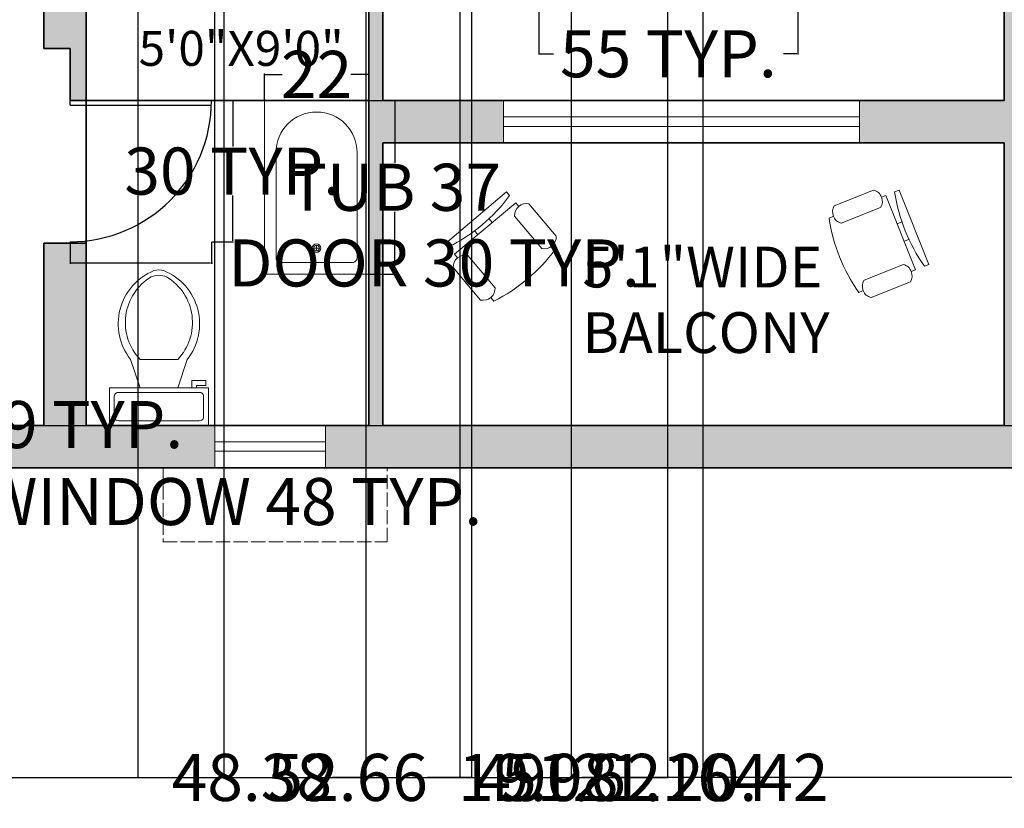
# Model space of a CAD drawing. Units: inches. Extents: x 300 to 1007, y 2 to 1069.
# Tile 2 of 12: x 557 to 766, y 2 to 170. Entities that reach past the tile are written whole.
import ezdxf

# ---------------------------------------------------------------- set-up
doc = ezdxf.new("R2010")
doc.units = ezdxf.units.IN
doc.header["$MEASUREMENT"] = 0
doc.linetypes.add('ACAD_ISO02W100', pattern=[15, 12, -3])
for name, color, linetype, lineweight in [('A-ANNO-DIMS', 2, 'Continuous', 18), ('A-AREA-IDEN', 7, 'Continuous', 18), ('A-DOOR', 3, 'Continuous', 25), ('A-FLOR-FIXT', 9, 'Continuous', 18), ('A-FURN', 8, 'Continuous', 18), ('A-GLAZ', 4, 'Continuous', 18), ('A-GLAZ-OVHD', 8, 'ACAD_ISO02W100', 13), ('A-WALL', 7, 'Continuous', 35)]:
    doc.layers.add(name, color=color, linetype=linetype, lineweight=lineweight)
doc.layers.add('A-WALL-PATT', color=9, linetype='Continuous', lineweight=9, true_color=0xc7c8ca)
doc.styles.get("Standard").update_dxf_attribs({"font": 'arial.ttf'})
doc.dimstyles.get("Standard").update_dxf_attribs({"dimtxt": 10, "dimasz": 0.18, "dimexe": 0.18, "dimexo": 0.0625, "dimgap": 0.09, "dimtad": 0, "dimtih": 1, "dimtoh": 1, "dimdec": 0, "dimzin": 0, "dimdsep": 46, "dimlunit": 3, "dimtxsty": 'Standard', "dimcen": 0.09, "dimadec": 0, "dimazin": 0, "dimtfac": 1, "dimtdec": 0, "dimtofl": 0, "dimtmove": 0, "dimatfit": 3, "dimfxl": 1, "dimtolj": 1, "dimtzin": 0, "dimarcsym": 0})

# ---------------------------------------------------------------- blocks, each defined once
blk = doc.blocks.new('Chair - Desk')
for p, q in [((-8.5, 0), (-8.5, -1)), ((-8.5, 0), (8.5, 0)), ((8.5, 0), (8.5, -1)), ((-2, -3), (-2, -1.9355)), ((2, -1.9576), (2, -3)), ((-8.5, -3), (-8.5, -4)), ((-8.5, -3), (8.5, -3)), ((8.5, -3), (8.5, -4)), ((-10.5, -5), (-10.5, -14)), ((-6.5, -14), (-6.5, -5)), ((6.5, -5), (6.5, -14)), ((10.5, -14), (10.5, -5)), ((-8.5, -15), (-8.5, -16)), ((8.5, -15), (8.5, -16))]:
    blk.add_line(p, q)
for centre, radius, start, end in [((0, 34.625), 36.625, 256.5803, 283.4197), ((-8.5, -6.5), 2.5, 36.8699, 143.1301), ((8.5, -6.5), 2.5, 36.8699, 143.1301), ((-8.5, -12.5), 2.5, 216.8699, 323.1301), ((8.5, -12.5), 2.5, 216.8699, 323.1301), ((0, 19.625), 36.625, 256.5803, 283.4197)]:
    blk.add_arc(centre, radius, start, end)
blk = doc.blocks.new('Toilet - top')
for p, q in [((9.5, -6), (9.5, -2)), ((-8, -8.5), (-8, -8)), ((-7, -8), (-7, -9.5)), ((-4, -8), (-6, -14)), ((4, -8), (6, -14)), ((-10, -8.5), (-8, -8.5)), ((-10, -9.5), (-10, -8.5)), ((-7, -9.5), (-10, -9.5)), ((4, -14), (-4, -14))]:
    blk.add_line(p, q)
blk.add_lwpolyline([(10.5, -8), (10.5, 0), (-10.5, 0), (-10.5, -8)], close=True)
for points in [[(-9.5, -2), (-9.5, -6)], [(8.5, -1), (-8.5, -1)], [(-8.5, -7), (8.5, -7)]]:
    blk.add_lwpolyline(points)
for centre, radius, start, end in [((-8.62, -1.88), 0.884, 81.8699, 188.1301), ((8.62, -1.88), 0.884, 351.8699, 98.1301), ((-8.62, -6.12), 0.884, 171.8699, 278.1301), ((8.62, -6.12), 0.884, 261.8699, 8.1301), ((3.52, -21.58), 12.17, 141.4691, 247.9714), ((4.2, -21.82), 11.33, 136.3677, 238.9468), ((-3.52, -21.58), 12.17, 292.0284, 38.5307), ((-4.2, -21.82), 11.33, 301.053, 43.6321), ((0, -27.88), 4, 245.7318, 294.2682), ((0, -29), 4, 254.8605, 285.1395)]:
    blk.add_arc(centre, radius, start, end)
blk = doc.blocks.new('Bath Tub - 26 x 60 in.')
for p, q in [((9, -17), (9, -19)), ((8, -18), (10, -18))]:
    blk.add_line(p, q)
blk.add_lwpolyline([(0, -36), (0, 0), (60, 0), (60, -36)], close=True)
for points in [[(4, -30), (4, -6)], [(6, -4), (42, -4)], [(42, -32), (6, -32)]]:
    blk.add_lwpolyline(points)
for radius in [1.5, 1]:
    blk.add_circle((9, -18), radius)
for centre, radius, start, end in [((5.75, -5.75), 1.77, 81.8699, 188.1301), ((42, -18), 14, 270, 90), ((5.75, -30.25), 1.77, 171.8699, 278.1301)]:
    blk.add_arc(centre, radius, start, end)
blk = doc.blocks.new('DOOR-SINGLE-30')
for p, q in [((0, 0), (30, 0)), ((0, -1), (0, 0)), ((0, -1), (30, -1))]:
    blk.add_line(p, q)
blk.add_arc((0, 0), 30, 270, 0)
blk = doc.blocks.new('*D33')
at = {"layer": 'A-ANNO-DIMS', "color": 0, "lineweight": -2, "transparency": 16777216}
for p, q in [((631.18, 152.38), (636.83, 152.38)), ((636.65, 152.2), (636.65, 139.14)), ((636.65, 115.69), (636.65, 128.75)), ((631.18, 115.51), (636.83, 115.51))]:
    blk.add_line(p, q, dxfattribs=at)
at = {"layer": 'A-ANNO-DIMS', "color": 0, "transparency": 16777216}
for points in [[(636.62, 152.2), (636.68, 152.2), (636.65, 152.38)], [(636.62, 115.69), (636.68, 115.69), (636.65, 115.51)]]:
    blk.add_solid(points, dxfattribs=at)
at = {"layer": 'Defpoints', "color": 0, "transparency": 16777216}
for p in [(631.12, 152.38), (636.65, 152.38), (631.12, 115.51)]:
    blk.add_point(p, dxfattribs=at)
at = {"layer": 'A-ANNO-DIMS', "color": 0, "transparency": 16777216, "insert": (636.65, 133.95), "char_height": 10, "attachment_point": 5}
blk.add_mtext('\\A1;TUB 37', dxfattribs=at)
blk = doc.blocks.new('*D34')
at = {"layer": 'A-ANNO-DIMS', "color": 0, "lineweight": -2, "transparency": 16777216}
for p, q in [((608.99, 152.45), (608.99, 158.1)), ((609.17, 157.92), (612.77, 157.92)), ((630.94, 157.92), (627.34, 157.92)), ((631.12, 152.45), (631.12, 158.1))]:
    blk.add_line(p, q, dxfattribs=at)
at = {"layer": 'A-ANNO-DIMS', "color": 0, "transparency": 16777216}
for points in [[(609.17, 157.95), (609.17, 157.89), (608.99, 157.92)], [(630.94, 157.95), (630.94, 157.89), (631.12, 157.92)]]:
    blk.add_solid(points, dxfattribs=at)
at = {"layer": 'Defpoints', "color": 0, "transparency": 16777216}
for p in [(608.99, 157.92), (608.99, 152.38), (631.12, 152.38)]:
    blk.add_point(p, dxfattribs=at)
at = {"layer": 'A-ANNO-DIMS', "color": 0, "transparency": 16777216, "insert": (620.06, 157.92), "char_height": 10, "attachment_point": 5}
blk.add_mtext('\\A1;22', dxfattribs=at)
blk = doc.blocks.new('*D43')
at = {"layer": 'A-ANNO-DIMS', "color": 0, "lineweight": -2, "transparency": 16777216}
for p, q in [((496.77, 74.32), (496.77, 67.03)), ((544.6, 74.32), (544.6, 67.03)), ((496.95, 67.21), (544.42, 67.21)), ((544.6, 67.21), (544.78, 67.21))]:
    blk.add_line(p, q, dxfattribs=at)
at = {"layer": 'A-ANNO-DIMS', "color": 0, "transparency": 16777216}
for points in [[(496.95, 67.24), (496.95, 67.18), (496.77, 67.21)], [(544.42, 67.24), (544.42, 67.18), (544.6, 67.21)]]:
    blk.add_solid(points, dxfattribs=at)
at = {"layer": 'Defpoints', "color": 0, "transparency": 16777216}
for p in [(496.77, 74.38), (544.6, 74.38), (544.6, 67.21)]:
    blk.add_point(p, dxfattribs=at)
at = {"layer": 'A-ANNO-DIMS', "color": 0, "transparency": 16777216, "insert": (602, 67.21), "char_height": 10, "attachment_point": 5}
blk.add_mtext('\\A1;WINDOW 48 TYP.', dxfattribs=at)
blk = doc.blocks.new('*D44')
at = {"layer": 'A-ANNO-DIMS', "color": 0, "lineweight": -2, "transparency": 16777216}
for p, q in [((544.67, 83.38), (551.96, 83.38)), ((551.78, 83.38), (551.78, 83.56)), ((551.78, 83.56), (551.96, 83.56)), ((551.78, 74.56), (551.78, 83.2)), ((544.67, 74.38), (551.96, 74.38))]:
    blk.add_line(p, q, dxfattribs=at)
at = {"layer": 'A-ANNO-DIMS', "color": 0, "transparency": 16777216}
for points in [[(551.75, 83.2), (551.81, 83.2), (551.78, 83.38)], [(551.75, 74.56), (551.81, 74.56), (551.78, 74.38)]]:
    blk.add_solid(points, dxfattribs=at)
at = {"layer": 'Defpoints', "color": 0, "transparency": 16777216}
for p in [(544.6, 83.38), (551.78, 83.38), (544.6, 74.38)]:
    blk.add_point(p, dxfattribs=at)
at = {"layer": 'A-ANNO-DIMS', "color": 0, "transparency": 16777216, "insert": (572.5, 83.56), "char_height": 10, "attachment_point": 5}
blk.add_mtext('\\A1;9 TYP.', dxfattribs=at)
blk = doc.blocks.new('*D54')
at = {"layer": 'A-ANNO-DIMS', "color": 0, "lineweight": -2, "transparency": 16777216}
for p, q in [((667.27, 175.9), (667.27, 162.13)), ((722.27, 175.9), (722.27, 162.13)), ((667.45, 162.31), (670.34, 162.31)), ((722.09, 162.31), (719.2, 162.31))]:
    blk.add_line(p, q, dxfattribs=at)
at = {"layer": 'A-ANNO-DIMS', "color": 0, "transparency": 16777216}
for points in [[(667.45, 162.34), (667.45, 162.28), (667.27, 162.31)], [(722.09, 162.34), (722.09, 162.28), (722.27, 162.31)]]:
    blk.add_solid(points, dxfattribs=at)
at = {"layer": 'Defpoints', "color": 0, "transparency": 16777216}
for p in [(667.27, 175.96), (722.27, 175.96), (722.27, 162.31)]:
    blk.add_point(p, dxfattribs=at)
at = {"layer": 'A-ANNO-DIMS', "color": 0, "transparency": 16777216, "insert": (694.77, 162.31), "char_height": 10, "attachment_point": 5}
blk.add_mtext('\\A1;55 TYP.', dxfattribs=at)
blk = doc.blocks.new('*D63')
at = {"layer": 'A-ANNO-DIMS', "color": 0, "lineweight": -2, "transparency": 16777216}
for p, q in [((567.74, 122.32), (567.74, 117.7)), ((597.74, 122.32), (597.74, 117.7)), ((567.92, 117.88), (597.56, 117.88)), ((597.74, 117.88), (597.92, 117.88))]:
    blk.add_line(p, q, dxfattribs=at)
at = {"layer": 'A-ANNO-DIMS', "color": 0, "transparency": 16777216}
for points in [[(567.92, 117.91), (567.92, 117.85), (567.74, 117.88)], [(597.56, 117.91), (597.56, 117.85), (597.74, 117.88)]]:
    blk.add_solid(points, dxfattribs=at)
at = {"layer": 'Defpoints', "color": 0, "transparency": 16777216}
for p in [(567.74, 122.38), (597.74, 122.38), (597.74, 117.88)]:
    blk.add_point(p, dxfattribs=at)
at = {"layer": 'A-ANNO-DIMS', "color": 0, "transparency": 16777216, "insert": (645, 117.88), "char_height": 10, "attachment_point": 5}
blk.add_mtext('\\A1;DOOR 30 TYP.', dxfattribs=at)
blk = doc.blocks.new('*D64')
at = {"layer": 'A-ANNO-DIMS', "color": 0, "lineweight": -2, "transparency": 16777216}
for p, q in [((597.8, 152.38), (602.42, 152.38)), ((602.24, 152.2), (602.24, 142.58)), ((602.24, 122.56), (602.24, 132.19)), ((597.8, 122.38), (602.42, 122.38))]:
    blk.add_line(p, q, dxfattribs=at)
at = {"layer": 'A-ANNO-DIMS', "color": 0, "transparency": 16777216}
for points in [[(602.21, 152.2), (602.27, 152.2), (602.24, 152.38)], [(602.21, 122.56), (602.27, 122.56), (602.24, 122.38)]]:
    blk.add_solid(points, dxfattribs=at)
at = {"layer": 'Defpoints', "color": 0, "transparency": 16777216}
for p in [(597.74, 152.38), (602.24, 152.38), (597.74, 122.38)]:
    blk.add_point(p, dxfattribs=at)
at = {"layer": 'A-ANNO-DIMS', "color": 0, "transparency": 16777216, "insert": (602.24, 137.38), "char_height": 10, "attachment_point": 5}
blk.add_mtext('\\A1;30 TYP.', dxfattribs=at)
blk = doc.blocks.new('*D73')
at = {"layer": 'A-ANNO-DIMS', "color": 0, "lineweight": -2, "transparency": 16777216}
for p, q in [((420.12, 74.32), (420.12, 8.45)), ((910.12, 74.32), (910.12, 8.45)), ((420.3, 8.63), (653.8, 8.63)), ((909.94, 8.63), (676.44, 8.63))]:
    blk.add_line(p, q, dxfattribs=at)
at = {"layer": 'A-ANNO-DIMS', "color": 0, "transparency": 16777216}
for points in [[(420.3, 8.66), (420.3, 8.6), (420.12, 8.63)], [(909.94, 8.66), (909.94, 8.6), (910.12, 8.63)]]:
    blk.add_solid(points, dxfattribs=at)
at = {"layer": 'Defpoints', "color": 0, "transparency": 16777216}
for p in [(420.12, 74.38), (910.12, 74.38), (910.12, 8.63)]:
    blk.add_point(p, dxfattribs=at)
at = {"layer": 'A-ANNO-DIMS', "color": 0, "transparency": 16777216, "insert": (665.12, 8.63), "char_height": 10, "attachment_point": 5}
blk.add_mtext('\\A1;490', dxfattribs=at)
blk = doc.blocks.new('*D89')
at = {"layer": 'A-ANNO-DIMS', "color": 0, "lineweight": -2, "transparency": 16777216}
for p, q in [((544.6, 83.45), (544.6, 1063.03)), ((544.78, 1062.85), (554.56, 1062.85)), ((598.25, 1062.85), (588.48, 1062.85)), ((598.43, 83.45), (598.43, 1063.03))]:
    blk.add_line(p, q, dxfattribs=at)
at = {"layer": 'A-ANNO-DIMS', "color": 0, "transparency": 16777216}
for points in [[(544.78, 1062.88), (544.78, 1062.82), (544.6, 1062.85)], [(598.25, 1062.88), (598.25, 1062.82), (598.43, 1062.85)]]:
    blk.add_solid(points, dxfattribs=at)
at = {"layer": 'Defpoints', "color": 0, "transparency": 16777216}
for p in [(598.43, 1062.85), (544.6, 83.38), (598.43, 83.38)]:
    blk.add_point(p, dxfattribs=at)
at = {"layer": 'A-ANNO-DIMS', "color": 0, "transparency": 16777216, "insert": (571.52, 1062.85), "char_height": 10, "attachment_point": 5}
blk.add_mtext('\\A1;53.83', dxfattribs=at)
blk = doc.blocks.new('*D90')
at = {"layer": 'A-ANNO-DIMS', "color": 0, "lineweight": -2, "transparency": 16777216}
for p, q in [((429.18, 209), (974.48, 209)), ((974.3, 208.82), (974.3, 151.39)), ((974.3, 83.56), (974.3, 141)), ((429.18, 83.38), (974.48, 83.38))]:
    blk.add_line(p, q, dxfattribs=at)
at = {"layer": 'A-ANNO-DIMS', "color": 0, "transparency": 16777216}
for points in [[(974.27, 208.82), (974.33, 208.82), (974.3, 209)], [(974.27, 83.56), (974.33, 83.56), (974.3, 83.38)]]:
    blk.add_solid(points, dxfattribs=at)
at = {"layer": 'Defpoints', "color": 0, "transparency": 16777216}
for p in [(429.12, 209), (974.3, 209), (429.12, 83.38)]:
    blk.add_point(p, dxfattribs=at)
at = {"layer": 'A-ANNO-DIMS', "color": 0, "transparency": 16777216, "insert": (974.3, 146.19), "char_height": 10, "attachment_point": 5}
blk.add_mtext('\\A1;125.61', dxfattribs=at)
blk = doc.blocks.new('*D102')
at = {"layer": 'A-ANNO-DIMS', "color": 0, "lineweight": -2, "transparency": 16777216}
for p, q in [((600.34, 609.38), (600.34, 8.45)), ((652.99, 609.38), (652.99, 8.45)), ((600.52, 8.63), (609.71, 8.63)), ((652.81, 8.63), (643.62, 8.63))]:
    blk.add_line(p, q, dxfattribs=at)
at = {"layer": 'A-ANNO-DIMS', "color": 0, "transparency": 16777216}
for points in [[(600.52, 8.66), (600.52, 8.6), (600.34, 8.63)], [(652.81, 8.66), (652.81, 8.6), (652.99, 8.63)]]:
    blk.add_solid(points, dxfattribs=at)
at = {"layer": 'Defpoints', "color": 0, "transparency": 16777216}
for p in [(600.34, 609.45), (652.99, 609.45), (652.99, 8.63)]:
    blk.add_point(p, dxfattribs=at)
at = {"layer": 'A-ANNO-DIMS', "color": 0, "transparency": 16777216, "insert": (626.66, 8.63), "char_height": 10, "attachment_point": 5}
blk.add_mtext('\\A1;52.66', dxfattribs=at)
blk = doc.blocks.new('*D103')
at = {"layer": 'A-ANNO-DIMS', "color": 0, "lineweight": -2, "transparency": 16777216}
for p, q in [((652.99, 609.38), (652.99, 8.45)), ((674.16, 609.38), (674.16, 8.45)), ((653.17, 8.63), (673.98, 8.63)), ((674.16, 8.63), (674.34, 8.63))]:
    blk.add_line(p, q, dxfattribs=at)
at = {"layer": 'A-ANNO-DIMS', "color": 0, "transparency": 16777216}
for points in [[(653.17, 8.66), (653.17, 8.6), (652.99, 8.63)], [(673.98, 8.66), (673.98, 8.6), (674.16, 8.63)]]:
    blk.add_solid(points, dxfattribs=at)
at = {"layer": 'Defpoints', "color": 0, "transparency": 16777216}
for p in [(652.99, 609.45), (674.16, 609.45), (674.16, 8.63)]:
    blk.add_point(p, dxfattribs=at)
at = {"layer": 'A-ANNO-DIMS', "color": 0, "transparency": 16777216, "insert": (695.25, 8.63), "char_height": 10, "attachment_point": 5}
blk.add_mtext('\\A1;21.164', dxfattribs=at)
blk = doc.blocks.new('*D104')
at = {"layer": 'A-ANNO-DIMS', "color": 0, "lineweight": -2, "transparency": 16777216}
for p, q in [((674.16, 609.38), (674.16, 8.45)), ((694.58, 609.38), (694.58, 8.45)), ((674.34, 8.63), (694.4, 8.63)), ((694.58, 8.63), (694.76, 8.63))]:
    blk.add_line(p, q, dxfattribs=at)
at = {"layer": 'A-ANNO-DIMS', "color": 0, "transparency": 16777216}
for points in [[(674.34, 8.66), (674.34, 8.6), (674.16, 8.63)], [(694.4, 8.66), (694.4, 8.6), (694.58, 8.63)]]:
    blk.add_solid(points, dxfattribs=at)
at = {"layer": 'Defpoints', "color": 0, "transparency": 16777216}
for p in [(674.16, 609.45), (694.58, 609.45), (694.58, 8.63)]:
    blk.add_point(p, dxfattribs=at)
at = {"layer": 'A-ANNO-DIMS', "color": 0, "transparency": 16777216, "insert": (711.75, 8.63), "char_height": 10, "attachment_point": 5}
blk.add_mtext('\\A1;20.42', dxfattribs=at)
blk = doc.blocks.new('*D106')
at = {"layer": 'A-ANNO-DIMS', "color": 0, "lineweight": -2, "transparency": 16777216}
for p, q in [((582.11, 990.38), (582.11, 8.45)), ((630.49, 990.38), (630.49, 8.45)), ((582.29, 8.63), (589.12, 8.63)), ((630.31, 8.63), (623.47, 8.63))]:
    blk.add_line(p, q, dxfattribs=at)
at = {"layer": 'A-ANNO-DIMS', "color": 0, "transparency": 16777216}
for points in [[(582.29, 8.66), (582.29, 8.6), (582.11, 8.63)], [(630.31, 8.66), (630.31, 8.6), (630.49, 8.63)]]:
    blk.add_solid(points, dxfattribs=at)
at = {"layer": 'Defpoints', "color": 0, "transparency": 16777216}
for p in [(582.11, 990.45), (630.49, 990.45), (630.49, 8.63)]:
    blk.add_point(p, dxfattribs=at)
at = {"layer": 'A-ANNO-DIMS', "color": 0, "transparency": 16777216, "insert": (606.3, 8.63), "char_height": 10, "attachment_point": 5}
blk.add_mtext('\\A1;48.38', dxfattribs=at)
blk = doc.blocks.new('*D107')
at = {"layer": 'A-ANNO-DIMS', "color": 0, "lineweight": -2, "transparency": 16777216}
for p, q in [((630.49, 990.38), (630.49, 8.45)), ((650.47, 990.38), (650.47, 8.45)), ((630.67, 8.63), (650.29, 8.63)), ((650.47, 8.63), (650.65, 8.63))]:
    blk.add_line(p, q, dxfattribs=at)
at = {"layer": 'A-ANNO-DIMS', "color": 0, "transparency": 16777216}
for points in [[(630.67, 8.66), (630.67, 8.6), (630.49, 8.63)], [(650.29, 8.66), (650.29, 8.6), (650.47, 8.63)]]:
    blk.add_solid(points, dxfattribs=at)
at = {"layer": 'Defpoints', "color": 0, "transparency": 16777216}
for p in [(630.49, 990.45), (650.47, 990.45), (650.47, 8.63)]:
    blk.add_point(p, dxfattribs=at)
at = {"layer": 'A-ANNO-DIMS', "color": 0, "transparency": 16777216, "insert": (667.15, 8.63), "char_height": 10, "attachment_point": 5}
blk.add_mtext('\\A1;19.98', dxfattribs=at)
blk = doc.blocks.new('*D108')
at = {"layer": 'A-ANNO-DIMS', "color": 0, "lineweight": -2, "transparency": 16777216}
for p, q in [((650.47, 990.38), (650.47, 8.45)), ((702.09, 990.38), (702.09, 8.45)), ((650.65, 8.63), (659.37, 8.63)), ((701.91, 8.63), (693.19, 8.63))]:
    blk.add_line(p, q, dxfattribs=at)
at = {"layer": 'A-ANNO-DIMS', "color": 0, "transparency": 16777216}
for points in [[(650.65, 8.66), (650.65, 8.6), (650.47, 8.63)], [(701.91, 8.66), (701.91, 8.6), (702.09, 8.63)]]:
    blk.add_solid(points, dxfattribs=at)
at = {"layer": 'Defpoints', "color": 0, "transparency": 16777216}
for p in [(650.47, 990.45), (702.09, 990.45), (702.09, 8.63)]:
    blk.add_point(p, dxfattribs=at)
at = {"layer": 'A-ANNO-DIMS', "color": 0, "transparency": 16777216, "insert": (676.28, 8.63), "char_height": 10, "attachment_point": 5}
blk.add_mtext('\\A1;51.62', dxfattribs=at)

msp = doc.modelspace()

# ---------------------------------------------------------------- hatches: boundary and pattern name
at = {"layer": 'A-WALL-PATT'}
h = msp.add_hatch(color=256, dxfattribs=at)
h.dxf.hatch_style = 1
h.paths.add_polyline_path([(546.104, 999.4468), (478.8267, 999.4468), (478.8267, 869.2798, -0.06322715), (487.8267, 868.1328), (487.8267, 990.4468), (546.104, 990.4468)])
h.paths.add_polyline_path([(630.4852, 999.4468), (582.106, 999.4468), (582.106, 990.4468), (613.8267, 990.4468), (613.8267, 867.4468), (622.8267, 867.4468), (622.8267, 990.4468), (630.4852, 990.4468)])
h.paths.add_polyline_path([(702.0883, 999.4468), (650.4653, 999.4468), (650.4653, 990.4468), (682.8267, 990.4468), (682.8267, 960.0824, -0.02530575), (685.8267, 960.0478), (685.8267, 990.4468), (702.0883, 990.4468)])
h.paths.add_polyline_path([(850.8267, 999.4468), (737.5888, 999.4468), (737.5888, 990.4468), (841.8267, 990.4468), (841.8267, 950.5685), (850.8267, 950.5685)])
h.paths.add_polyline_path([(685.8267, 930.4465), (682.8267, 930.4465), (682.8267, 888.4468), (682.8267, 867.4468), (685.8267, 867.4468), (697.4169, 867.4468), (697.4169, 870.4468), (685.8267, 870.4468), (685.8267, 888.4468)])
h.paths.add_polyline_path([(682.8267, 931.4465), (654.3436, 931.4465, 0.00843109), (654.3267, 930.4465), (682.8267, 930.4465)])
h.paths.add_polyline_path([(685.8267, 931.4465), (682.8267, 931.4465), (682.8267, 930.4465), (685.8267, 930.4465)])
h.paths.add_polyline_path([(682.8267, 888.4468), (622.8267, 888.4468), (622.8267, 885.4468), (682.8267, 885.4468)])
h.paths.add_polyline_path([(850.8267, 870.4468), (850.8267, 914.7851), (841.8267, 914.7851), (841.8267, 870.4468), (732.7101, 870.4468, -0.02120595), (732.8267, 867.4468), (779.8267, 867.4468), (779.8267, 749.4468), (782.8267, 749.4468), (788.8267, 749.4468), (788.8267, 861.4468), (841.8267, 861.4468), (841.8267, 749.4468), (850.8267, 749.4468)])
h.paths.add_polyline_path([(622.8267, 810.4468), (487.8267, 810.4468), (487.8267, 833.2626), (478.8267, 833.2626), (478.8267, 609.4468), (478.8267, 482.3847), (487.8267, 482.3847), (487.8267, 801.4468), (620.8267, 801.4468), (622.8267, 801.4468)])
h.paths.add_polyline_path([(680.8267, 729.4468), (620.8267, 729.4468), (620.8267, 765.8246, -0.02111352), (617.8267, 766.0562), (617.8267, 698.7303), (620.8267, 698.7303), (620.8267, 726.4468), (680.8267, 726.4468)])
h.paths.add_polyline_path([(620.8267, 668.8122, -0.02498293), (617.8267, 668.6448), (617.8267, 618.4468), (600.3357, 618.4468), (600.3357, 609.4468), (652.9929, 609.4468), (652.9929, 618.4468), (620.8267, 618.4468)])
h.paths.add_polyline_path([(552.3393, 618.4468), (487.8267, 618.4468), (487.8267, 609.4468), (552.3393, 609.4468)], flags=17)
h.paths.add_polyline_path([(694.5763, 618.4468), (683.8267, 618.4468), (683.8267, 726.4468), (683.8267, 749.4468), (680.8267, 749.4468), (680.8267, 740.4468), (680.8267, 726.4468), (680.8267, 618.4468), (674.1573, 618.4468), (674.1573, 609.4468), (680.8267, 609.4468), (694.5763, 609.4468)])
h.paths.add_polyline_path([(850.8267, 642.8902), (841.8267, 642.8902), (841.8267, 618.4468), (782.8267, 618.4468), (782.8267, 708.0513, -0.02308839), (779.8267, 707.9092), (779.8267, 618.4468), (730.1068, 618.4468), (730.1068, 609.4468), (779.8267, 609.4468), (841.8267, 609.4468), (841.8267, 482.3847), (850.8267, 482.3847)])
h.paths.add_polyline_path([(850.8267, 749.4468), (841.8267, 749.4468), (841.8267, 705.9119), (850.8267, 705.9119)])
h.paths.add_polyline_path([(841.8267, 749.4468), (782.8267, 749.4468), (779.8267, 749.4468), (761.9959, 749.4468), (761.9959, 740.4468), (779.8267, 740.4468), (812.3267, 740.4468), (841.8267, 740.4468)])
h.paths.add_polyline_path([(669.1457, 482.3847), (604.489, 482.3847), (604.489, 473.3847), (631.1217, 473.3847), (631.1217, 436.0244, -0.02504709), (634.1217, 436.1748), (634.1217, 436.4367), (634.1217, 473.3847), (669.1457, 473.3847)], flags=17)
h.paths.add_polyline_path([(580.5305, 482.3847), (571.1217, 482.3847), (541.0813, 482.3847), (541.0813, 473.3847), (562.1217, 473.3847), (562.1217, 326.3847), (571.1217, 326.3847), (571.1217, 362.3847), (631.1217, 362.3847), (631.1217, 326.3847), (706.9024, 326.3847, -0.02105388), (706.9999, 329.3847), (634.1217, 329.3847), (634.1217, 365.3847), (634.1217, 406.1748), (631.1217, 406.1748), (631.1217, 365.3847), (571.1217, 365.3847), (571.1217, 473.3847), (580.5305, 473.3847)])
h.paths.add_polyline_path([(493.4756, 482.3847), (420.1217, 482.3847), (420.1217, 445.3134), (429.1217, 445.3134), (429.1217, 473.3847), (493.4756, 473.3847)])
h.paths.add_polyline_path([(786.2236, 482.3847), (716.7793, 482.3847), (716.7793, 473.3847), (766.1217, 473.3847), (766.1217, 329.3847), (742.5583, 329.3847), (742.5583, 326.3847), (766.1217, 326.3847), (766.1217, 316.0647), (769.1217, 316.0647), (769.1217, 326.3847), (769.1217, 473.3847), (786.2236, 473.3847)])
h.paths.add_polyline_path([(910.1217, 482.3847), (822.7166, 482.3847), (822.7166, 473.3847), (901.1217, 473.3847), (901.1217, 402.5393), (910.1217, 402.5393)])
h.paths.add_polyline_path([(910.1217, 366.1034), (901.1217, 366.1034), (901.1217, 329.3847), (814.1217, 329.3847), (814.1217, 312.5176), (817.1217, 312.5176), (817.1217, 326.3847), (901.1217, 326.3847), (901.1217, 293.0319), (910.1217, 293.0319), (910.1217, 326.3847)])
h.paths.add_polyline_path([(910.1217, 268.9355), (901.1217, 268.9355), (901.1217, 254.3847), (817.1217, 254.3847), (817.1217, 290.5411, -0.03396715), (814.1217, 290.3847), (814.1217, 254.3847), (775.1217, 254.3847), (775.1217, 281.5164), (769.1217, 281.5164), (769.1217, 292.1577), (766.1217, 292.1577), (766.1217, 254.3847), (766.1217, 220.1938), (775.5079, 220.1938), (775.5079, 251.3847), (817.1217, 251.3847), (901.1217, 251.3847), (901.1217, 152.3847), (819.0246, 152.3847, -0.02493798), (818.9117, 149.3847), (901.1217, 149.3847), (901.1217, 92.3847), (901.1217, 83.3847), (874.3528, 83.3847), (874.3528, 74.3847), (910.1217, 74.3847), (910.1217, 92.3847), (910.1217, 149.3847)])
h.paths.add_polyline_path([(429.1217, 325.0924), (420.1217, 325.0924), (420.1217, 263.3847), (420.1217, 244.9834), (429.1217, 244.9834), (429.1217, 269.3847), (571.1217, 269.3847), (571.1217, 272.3847), (562.1217, 272.3847), (429.1217, 272.3847)])
h.paths.add_polyline_path([(429.1217, 208.998), (420.1217, 208.998), (420.1217, 74.3847), (496.7704, 74.3847), (496.7704, 83.3847), (429.1217, 83.3847)])
h.paths.add_polyline_path([(598.4322, 83.3847), (571.1217, 83.3847), (571.1217, 122.1171), (562.1217, 122.1171), (562.1217, 83.3847), (544.6031, 83.3847), (544.6031, 74.3847), (598.4322, 74.3847)])
h.paths.add_polyline_path([(797.0822, 83.3847), (769.1217, 83.3847), (769.1217, 149.3847), (788.9123, 149.3847), (788.9123, 152.3847), (769.1217, 152.3847), (769.1217, 178.0167), (766.1217, 178.0167), (766.1217, 152.3847), (735.3598, 152.3847), (735.3598, 143.3847), (766.1217, 143.3847), (766.1217, 83.3847), (634.1217, 83.3847), (634.1217, 143.3847), (659.7326, 143.3847), (659.7326, 152.3847), (634.1217, 152.3847), (634.1217, 194.3847), (571.1217, 194.3847), (571.1217, 233.7289, -0.06379947), (562.1217, 234.7942), (562.1217, 163.4485), (567.7403, 163.4485), (567.7403, 152.3847), (571.1217, 152.3847), (571.1217, 191.3847), (631.1217, 191.3847), (631.1217, 83.3847), (621.979, 83.3847), (621.979, 74.3847), (631.1217, 74.3847), (797.0822, 74.3847)])

# ---------------------------------------------------------------- linework, layer by layer
at = {"layer": 'A-DOOR'}
msp.add_line((567.7403, 122.3847), (567.7403, 122.1171), dxfattribs=at)
at = {"layer": 'A-GLAZ'}
for p, q in [((659.7326, 152.3847), (659.7326, 143.3847)), ((735.3598, 152.3847), (735.3598, 143.3847)), ((659.7326, 148.8847), (735.3598, 148.8847)), ((659.7326, 146.8847), (735.3598, 146.8847)), ((598.4322, 78.8847), (598.4322, 83.3847)), ((598.4322, 83.3847), (598.4322, 74.3847)), ((621.979, 83.3847), (621.979, 74.3847)), ((621.979, 79.8847), (598.4322, 79.8847)), ((621.979, 77.8847), (598.4322, 77.8847))]:
    msp.add_line(p, q, dxfattribs=at)
at = {"layer": 'A-GLAZ-OVHD', "ltscale": 0.25}
for p, q in [((587.4374, 74.3847), (587.4374, 58.6606)), ((635.0299, 58.6606), (635.0299, 74.3847)), ((587.4374, 58.6606), (635.0299, 58.6606))]:
    msp.add_line(p, q, dxfattribs=at)
at = {"layer": 'A-WALL'}
for p, q in [((562.1217, 163.4485), (562.1217, 234.7942)), ((634.1217, 152.3847), (634.1217, 194.3847)), ((571.1217, 83.3847), (571.1217, 191.3847)), ((631.1217, 83.3847), (631.1217, 191.3847)), ((766.1217, 152.3847), (766.1217, 178.0167)), ((562.1217, 163.4485), (567.7403, 163.4485)), ((567.7403, 163.4485), (567.7403, 152.3847)), ((631.1217, 152.3847), (567.7403, 152.3847)), ((766.1217, 152.3847), (634.1217, 152.3847)), ((634.1217, 83.3847), (634.1217, 143.3847)), ((766.1217, 143.3847), (634.1217, 143.3847)), ((766.1217, 143.3847), (766.1217, 83.3847)), ((562.1217, 83.3847), (562.1217, 122.1171)), ((562.1217, 122.1171), (571.1217, 122.1171)), ((429.1217, 83.3847), (562.1217, 83.3847)), ((571.1217, 83.3847), (631.1217, 83.3847)), ((634.1217, 83.3847), (766.1217, 83.3847)), ((420.1217, 74.3847), (910.1217, 74.3847)), ((571.1217, 74.3847), (631.1217, 74.3847)), ((631.1217, 74.3847), (910.1217, 74.3847))]:
    msp.add_line(p, q, dxfattribs=at)

# ---------------------------------------------------------------- block references
at = {"layer": 'A-DOOR'}
msp.add_blockref('DOOR-SINGLE-30', (567.7403, 152.3847), dxfattribs=at)
at = {"layer": 'A-FLOR-FIXT', "xscale": 0.6146362971528592, "yscale": 0.6146362971528592, "zscale": 0.6146362971528592, "rotation": 90}
msp.add_blockref('Bath Tub - 26 x 60 in.', (608.9948, 115.5065), dxfattribs=at)
at = {"layer": 'A-FLOR-FIXT', "rotation": 180}
msp.add_blockref('Toilet - top', (586.5678, 83.3847), dxfattribs=at)
at = {"layer": 'A-FURN'}
for p, rotation in [((653.9081, 127.4846), 40.09798961394616), ((746.9168, 125.4597), 291.8014092022638)]:
    msp.add_blockref('Chair - Desk', p, dxfattribs=dict(at, rotation=rotation))

# ---------------------------------------------------------------- texts
at = {"layer": 'A-AREA-IDEN'}
for s, height, p in [('5\'0"X9\'0"', 7.43087, (582.2535, 159.7285)), ('5\'1"WIDE', 8.66705, (676.5204, 112.6762)), ('BALCONY', 8.66705, (676.5204, 98.7533))]:
    msp.add_text(s, height=height, dxfattribs=at).set_placement(p)

# ---------------------------------------------------------------- dimensions: what is measured, and where the dimension line sits
at = {"layer": 'A-ANNO-DIMS'}
for base, p1, p2, override, picture, middle in [((598.4322, 1062.8469), (544.6031, 83.3847), (598.4322, 83.3847), {"dimdec": 2, "dimlfac": 1, "dimrnd": 0, "dimzin": 0, "dimdsep": 46, "dimlunit": 2}, '*D89', (571.5176, 1062.8469)), ((630.4852, 8.6288), (582.106, 990.4468), (630.4852, 990.4468), {"dimdec": 2, "dimlfac": 1, "dimrnd": 0, "dimzin": 0, "dimdsep": 46, "dimlunit": 2}, '*D106', (606.2956, 8.6288)), ((650.4653, 8.6288), (630.4852, 990.4468), (650.4653, 990.4468), {"dimdec": 2, "dimlfac": 1, "dimrnd": 0, "dimzin": 0, "dimdsep": 46, "dimlunit": 2}, '*D107', (667.1473, 8.6288)), ((702.0883, 8.6288), (650.4653, 990.4468), (702.0883, 990.4468), {"dimdec": 2, "dimlfac": 1, "dimrnd": 0, "dimzin": 0, "dimdsep": 46, "dimlunit": 2}, '*D108', (676.2768, 8.6288)), ((652.9929, 8.6288), (600.3357, 609.4468), (652.9929, 609.4468), {"dimdec": 2, "dimlfac": 1, "dimrnd": 0, "dimzin": 0, "dimdsep": 46, "dimlunit": 2}, '*D102', (626.6643, 8.6288)), ((674.1573, 8.6288), (652.9929, 609.4468), (674.1573, 609.4468), {"dimdec": 3, "dimlfac": 1, "dimrnd": 0, "dimzin": 0, "dimdsep": 46, "dimlunit": 2}, '*D103', (695.2493, 8.6288)), ((694.5763, 8.6288), (674.1573, 609.4468), (694.5763, 609.4468), {"dimdec": 2, "dimlfac": 1, "dimrnd": 0, "dimzin": 0, "dimdsep": 46, "dimlunit": 2}, '*D104', (711.7529, 8.6288)), ((910.1217, 8.6288), (420.1217, 74.3847), (910.1217, 74.3847), {"dimdec": 0, "dimlfac": 1, "dimrnd": 0, "dimzin": 0, "dimdsep": 46, "dimlunit": 2}, '*D73', (665.1217, 8.6288))]:
    dim = msp.add_linear_dim(base=base, p1=p1, p2=p2, dimstyle='Standard', override=override, dxfattribs=at)
    dim.commit()
    dim.dimension.update_dxf_attribs({"geometry": picture, "text_midpoint": middle})
for base, p1, p2, angle, override, picture, middle in [((974.3023, 208.998), (429.1217, 83.3847), (429.1217, 208.998), 90, {"dimdec": 2, "dimlfac": 1, "dimrnd": 0, "dimzin": 0, "dimdsep": 46, "dimlunit": 2}, '*D90', (974.3023, 146.1913)), ((608.9948, 157.9165), (631.1217, 152.3847), (608.9948, 152.3847), 180, {"dimdec": 0, "dimlfac": 1, "dimrnd": 0, "dimzin": 0, "dimdsep": 46, "dimlunit": 2}, '*D34', (620.0583, 157.9165))]:
    dim = msp.add_linear_dim(base=base, p1=p1, p2=p2, angle=angle, dimstyle='Standard', override=override, dxfattribs=at)
    dim.commit()
    dim.dimension.update_dxf_attribs({"geometry": picture, "text_midpoint": middle})
for base, p1, p2, text, picture, middle in [((722.2726, 162.3103), (667.2726, 175.9603), (722.2726, 175.9603), '<> TYP.', '*D54', (694.7726, 162.3103)), ((597.7403, 117.8847), (567.7403, 122.3847), (597.7403, 122.3847), 'DOOR <> TYP.', '*D63', (644.9953, 117.8847)), ((544.6031, 67.2098), (496.7704, 74.3847), (544.6031, 74.3847), 'WINDOW <> TYP.', '*D43', (602.0047, 67.2098))]:
    dim = msp.add_linear_dim(base=base, p1=p1, p2=p2, text=text, dimstyle='Standard', override={"dimdec": 0, "dimlfac": 1, "dimrnd": 0, "dimzin": 0, "dimdsep": 46, "dimlunit": 2}, dxfattribs=at)
    dim.commit()
    dim.dimension.update_dxf_attribs({"geometry": picture, "text_midpoint": middle})
for base, p1, p2, text, picture, middle in [((602.2403, 152.3847), (597.7403, 122.3847), (597.7403, 152.3847), '<> TYP.', '*D64', (602.2403, 137.3847)), ((636.6534, 152.3847), (631.1217, 115.5065), (631.1217, 152.3847), 'TUB <>', '*D33', (636.6534, 133.9456)), ((551.778, 83.3847), (544.6031, 74.3847), (544.6031, 83.3847), '<> TYP.', '*D44', (572.5016, 83.5647))]:
    dim = msp.add_linear_dim(base=base, p1=p1, p2=p2, angle=90, text=text, dimstyle='Standard', override={"dimdec": 0, "dimlfac": 1, "dimrnd": 0, "dimzin": 0, "dimdsep": 46, "dimlunit": 2}, dxfattribs=at)
    dim.commit()
    dim.dimension.update_dxf_attribs({"geometry": picture, "text_midpoint": middle})

doc.saveas('drawing.dxf')
